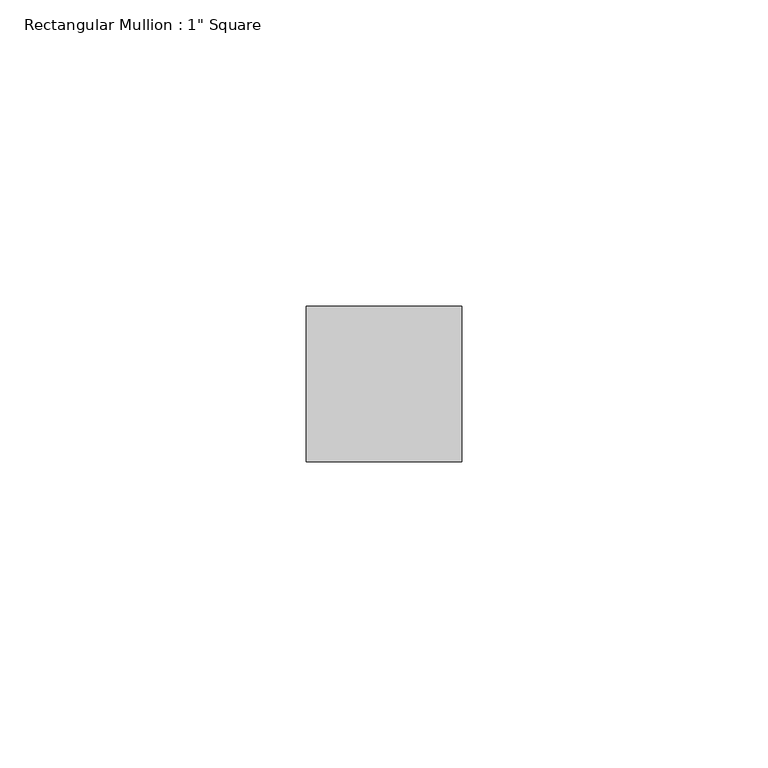
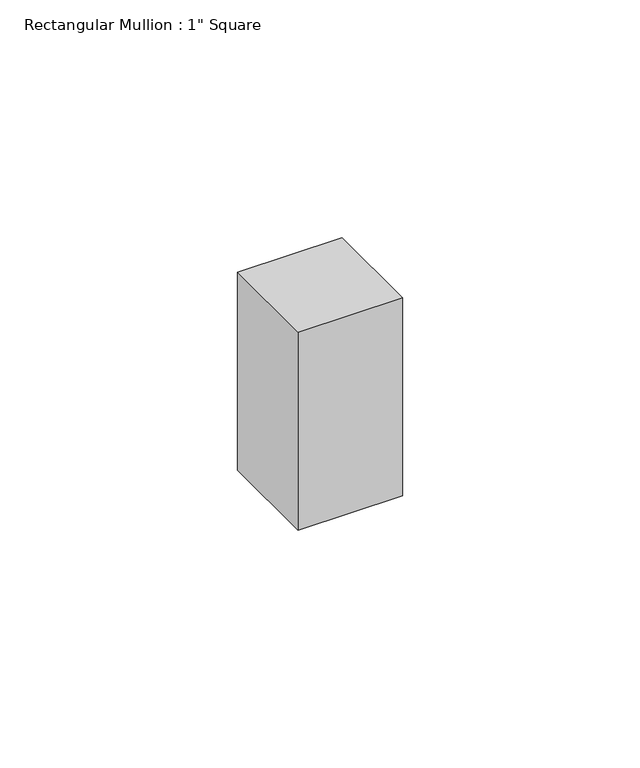
"""IFC4 building model written with IfcOpenShell, lengths in millimetres: member geometry."""

from ifc_helpers import new_model, si_unit, frame, origin, place, context, project, spatial, polyline, outline, extrude, source, transform, mapped, element, save


def member_06b3b9e2(model_context):
    return source(origin(), model_context, "Body", "SweptSolid", [
        extrude(outline(polyline([(0.0, 12.7), (0.0, -12.7), (-25.4, -12.7), (-25.4, 12.7), (0.0, 12.7)])), frame((0.0, 0.0, -50.8), z_axis=(0.0, 0.0, 1.0), x_axis=(1.0, 0.0, 0.0)), (0.0, 0.0, 1.0), 50.8),
    ])


if __name__ == "__main__":
    model = new_model("IFC4")
    model_context = context("Model", 3, world=origin())
    ifc_project = project(units=[si_unit("LENGTHUNIT", "METRE", prefix="MILLI")], contexts=[model_context])
    site = spatial("IfcSite", under=ifc_project)
    building = spatial("IfcBuilding", under=site)
    placement = place(None, origin())
    member_shape = member_06b3b9e2(model_context)
    element("IfcMember", 1, ObjectType="Rectangular Mullion : 1\" Square", at=placement, inside=building, context=model_context, shape_type="MappedRepresentation", body=[
        mapped(member_shape, transform((0.0, 0.0, 0.0), x_axis=(1.0, 0.0, 0.0), y_axis=(0.0, 1.0, 0.0), z_axis=(0.0, 0.0, 1.0))),
    ])
    save(model, "model.ifc")

# Revit data of these elements
# Type "Rectangular Mullion : 1\" Square"
#   built-in parameter 1007304 = 0.0833333 (stored number, unit not read)
#   built-in parameter 1007301 = 0.0416667 (stored number, unit not read)
#   built-in parameter 1007300 = 0.0416667 (stored number, unit not read)
# Element 1 (IfcMember, "Rectangular Mullion : 1\" Square")
#   Materials on its faces: "black"
# Materials
#   "black": class "Generic", colour RGB 120 120 120, transparency 0, Cost = 0
